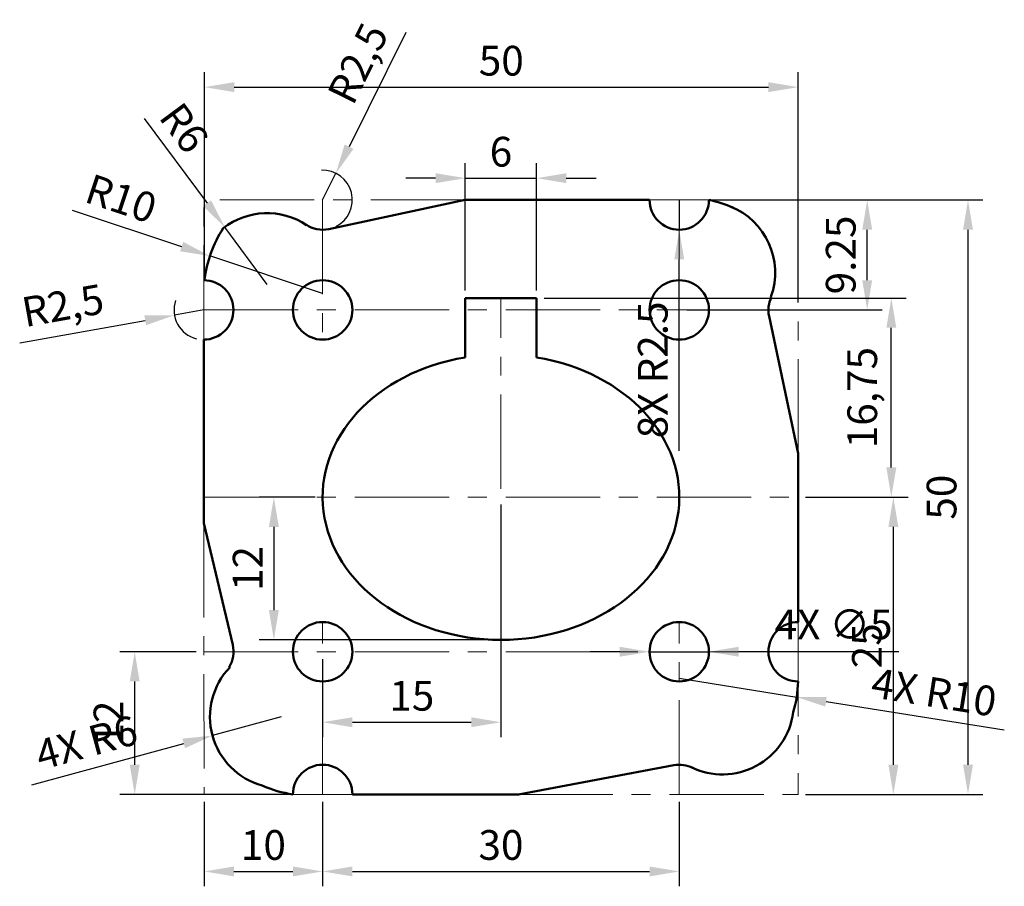
# Model space of a CAD drawing. Units: millimetres. Extents: x 2178 to 2260.8, y 1950.5 to 2023.4.
import ezdxf

# ---------------------------------------------------------------- set-up
doc = ezdxf.new("R2010")
doc.units = ezdxf.units.MM
doc.linetypes.add('CENTER', pattern=[50.8, 31.75, -6.35, 6.35, -6.35])
for name, color, linetype, lineweight in [('M-CNTR', 4, 'CENTER', 18), ('M-CONS', 8, 'CENTER', 13), ('M-DIMS', 2, 'Continuous', 25), ('M-OUTL', 7, 'Continuous', 50)]:
    doc.layers.add(name, color=color, linetype=linetype, lineweight=lineweight)
doc.styles.get("Standard").update_dxf_attribs({"font": 'arial.ttf'})
doc.dimstyles.new('ISO-25', dxfattribs={"dimtxt": 2.5, "dimasz": 2.5, "dimexe": 1.25, "dimexo": 0.625, "dimtad": 1, "dimtxsty": 'Standard', "dimcen": 2.5, "dimadec": 0, "dimazin": 0, "dimtfac": 1, "dimtmove": 0, "dimatfit": 3, "dimfxl": 1, "dimarcsym": 0})

# ---------------------------------------------------------------- blocks, each defined once
blk = doc.blocks.new('*D1')
at = {"layer": 'Defpoints', "color": 0, "transparency": 16777216}
for p in [(2221.441, 2010.03), (2215.441, 1999.949), (2221.441, 1999.949)]:
    blk.add_point(p, dxfattribs=at)
at = {"layer": 'M-DIMS', "color": 0, "lineweight": -2, "transparency": 16777216}
for p, q in [((2215.441, 2000.574), (2215.441, 2011.28)), ((2221.441, 2000.574), (2221.441, 2011.28)), ((2212.941, 2010.03), (2210.441, 2010.03)), ((2215.441, 2010.03), (2221.441, 2010.03)), ((2223.941, 2010.03), (2226.441, 2010.03))]:
    blk.add_line(p, q, dxfattribs=at)
at = {"layer": 'M-DIMS', "color": 0, "transparency": 16777216}
for points in [[(2212.941, 2010.447), (2212.941, 2009.613), (2215.441, 2010.03)], [(2223.941, 2010.447), (2223.941, 2009.613), (2221.441, 2010.03)]]:
    blk.add_solid(points, dxfattribs=at)
at = {"layer": 'M-DIMS', "color": 0, "transparency": 16777216, "insert": (2218.441, 2011.931), "char_height": 2.5, "attachment_point": 5}
blk.add_mtext('6', dxfattribs=at)
blk = doc.blocks.new('*D2')
at = {"layer": 'Defpoints', "color": 0, "transparency": 16777216}
for p in [(2243.441, 2017.687), (2193.504, 2001.448), (2243.441, 1998.949)]:
    blk.add_point(p, dxfattribs=at)
at = {"layer": 'M-DIMS', "color": 0, "lineweight": -2, "transparency": 16777216}
for p, q in [((2193.504, 2002.073), (2193.504, 2018.937)), ((2243.441, 1999.574), (2243.441, 2018.937)), ((2196.004, 2017.687), (2240.941, 2017.687))]:
    blk.add_line(p, q, dxfattribs=at)
at = {"layer": 'M-DIMS', "color": 0, "transparency": 16777216}
for points in [[(2196.004, 2018.104), (2196.004, 2017.27), (2193.504, 2017.687)], [(2240.941, 2018.104), (2240.941, 2017.27), (2243.441, 2017.687)]]:
    blk.add_solid(points, dxfattribs=at)
at = {"layer": 'M-DIMS', "color": 0, "transparency": 16777216, "insert": (2218.472, 2019.588), "char_height": 2.5, "attachment_point": 5}
blk.add_mtext('50', dxfattribs=at)
blk = doc.blocks.new('*D3')
at = {"layer": 'Defpoints', "color": 0, "transparency": 16777216}
for p in [(2203.441, 1983.199), (2199.34, 1971.199), (2218.441, 1971.199)]:
    blk.add_point(p, dxfattribs=at)
at = {"layer": 'M-DIMS', "color": 0, "lineweight": -2, "transparency": 16777216}
for p, q in [((2202.816, 1983.199), (2198.09, 1983.199)), ((2199.34, 1980.699), (2199.34, 1973.699)), ((2217.816, 1971.199), (2198.09, 1971.199))]:
    blk.add_line(p, q, dxfattribs=at)
at = {"layer": 'M-DIMS', "color": 0, "transparency": 16777216}
for points in [[(2198.923, 1980.699), (2199.756, 1980.699), (2199.34, 1983.199)], [(2198.923, 1973.699), (2199.756, 1973.699), (2199.34, 1971.199)]]:
    blk.add_solid(points, dxfattribs=at)
at = {"layer": 'M-DIMS', "color": 0, "transparency": 16777216, "insert": (2197.46, 1977.199), "char_height": 2.5, "attachment_point": 5, "rotation": 90}
blk.add_mtext('12', dxfattribs=at)
blk = doc.blocks.new('*D4')
at = {"layer": 'Defpoints', "color": 0, "transparency": 16777216}
for p in [(2218.441, 1983.199), (2203.441, 1970.199), (2218.441, 1964.27)]:
    blk.add_point(p, dxfattribs=at)
at = {"layer": 'M-DIMS', "color": 0, "lineweight": -2, "transparency": 16777216}
for p, q in [((2218.441, 1982.574), (2218.441, 1963.02)), ((2203.441, 1969.574), (2203.441, 1963.02)), ((2205.941, 1964.27), (2215.941, 1964.27))]:
    blk.add_line(p, q, dxfattribs=at)
at = {"layer": 'M-DIMS', "color": 0, "transparency": 16777216}
for points in [[(2205.941, 1964.687), (2205.941, 1963.853), (2203.441, 1964.27)], [(2215.941, 1964.687), (2215.941, 1963.853), (2218.441, 1964.27)]]:
    blk.add_solid(points, dxfattribs=at)
at = {"layer": 'M-DIMS', "color": 0, "transparency": 16777216, "insert": (2210.941, 1966.171), "char_height": 2.5, "attachment_point": 5}
blk.add_mtext('15', dxfattribs=at)
blk = doc.blocks.new('*D5')
at = {"layer": 'Defpoints', "color": 0, "transparency": 16777216}
for p in [(2193.477, 1958.199), (2203.441, 1958.199), (2203.441, 1951.721)]:
    blk.add_point(p, dxfattribs=at)
at = {"layer": 'M-DIMS', "color": 0, "lineweight": -2, "transparency": 16777216}
for p, q in [((2193.477, 1957.574), (2193.477, 1950.471)), ((2203.441, 1957.574), (2203.441, 1950.471)), ((2195.977, 1951.721), (2200.941, 1951.721))]:
    blk.add_line(p, q, dxfattribs=at)
at = {"layer": 'M-DIMS', "color": 0, "transparency": 16777216}
for points in [[(2195.977, 1952.138), (2195.977, 1951.305), (2193.477, 1951.721)], [(2200.941, 1952.138), (2200.941, 1951.305), (2203.441, 1951.721)]]:
    blk.add_solid(points, dxfattribs=at)
at = {"layer": 'M-DIMS', "color": 0, "transparency": 16777216, "insert": (2198.459, 1953.623), "char_height": 2.5, "attachment_point": 5}
blk.add_mtext('10', dxfattribs=at)
blk = doc.blocks.new('*D6')
at = {"layer": 'Defpoints', "color": 0, "transparency": 16777216}
for p in [(2203.441, 1958.199), (2233.441, 1958.199), (2233.441, 1951.721)]:
    blk.add_point(p, dxfattribs=at)
at = {"layer": 'M-DIMS', "color": 0, "lineweight": -2, "transparency": 16777216}
for p, q in [((2203.441, 1957.574), (2203.441, 1950.471)), ((2233.441, 1957.574), (2233.441, 1950.471)), ((2205.941, 1951.721), (2230.941, 1951.721))]:
    blk.add_line(p, q, dxfattribs=at)
at = {"layer": 'M-DIMS', "color": 0, "transparency": 16777216}
for points in [[(2205.941, 1952.138), (2205.941, 1951.305), (2203.441, 1951.721)], [(2230.941, 1952.138), (2230.941, 1951.305), (2233.441, 1951.721)]]:
    blk.add_solid(points, dxfattribs=at)
at = {"layer": 'M-DIMS', "color": 0, "transparency": 16777216, "insert": (2218.441, 1953.623), "char_height": 2.5, "attachment_point": 5}
blk.add_mtext('30', dxfattribs=at)
blk = doc.blocks.new('*D7')
at = {"layer": 'Defpoints', "color": 0, "transparency": 16777216}
for p in [(2243.441, 1983.199), (2251.45, 1983.199), (2243.441, 1958.199)]:
    blk.add_point(p, dxfattribs=at)
at = {"layer": 'M-DIMS', "color": 0, "lineweight": -2, "transparency": 16777216}
for p, q in [((2244.066, 1983.199), (2252.7, 1983.199)), ((2251.45, 1960.699), (2251.45, 1980.699)), ((2244.066, 1958.199), (2252.7, 1958.199))]:
    blk.add_line(p, q, dxfattribs=at)
at = {"layer": 'M-DIMS', "color": 0, "transparency": 16777216}
for points in [[(2251.033, 1980.699), (2251.867, 1980.699), (2251.45, 1983.199)], [(2251.033, 1960.699), (2251.867, 1960.699), (2251.45, 1958.199)]]:
    blk.add_solid(points, dxfattribs=at)
at = {"layer": 'M-DIMS', "color": 0, "transparency": 16777216, "insert": (2249.549, 1970.699), "char_height": 2.5, "attachment_point": 5, "rotation": 90}
blk.add_mtext('25', dxfattribs=at)
blk = doc.blocks.new('*D8')
at = {"layer": 'Defpoints', "color": 0, "transparency": 16777216}
for p in [(2221.441, 1999.949), (2251.28, 1999.949), (2243.441, 1983.199)]:
    blk.add_point(p, dxfattribs=at)
at = {"layer": 'M-DIMS', "color": 0, "lineweight": -2, "transparency": 16777216}
for p, q in [((2222.066, 1999.949), (2252.53, 1999.949)), ((2251.28, 1985.699), (2251.28, 1997.449)), ((2244.066, 1983.199), (2252.53, 1983.199))]:
    blk.add_line(p, q, dxfattribs=at)
at = {"layer": 'M-DIMS', "color": 0, "transparency": 16777216}
for points in [[(2250.864, 1997.449), (2251.697, 1997.449), (2251.28, 1999.949)], [(2250.864, 1985.699), (2251.697, 1985.699), (2251.28, 1983.199)]]:
    blk.add_solid(points, dxfattribs=at)
at = {"layer": 'M-DIMS', "color": 0, "transparency": 16777216, "insert": (2249.153, 1991.574), "char_height": 2.5, "attachment_point": 5, "rotation": 90}
blk.add_mtext('16,75', dxfattribs=at)
blk = doc.blocks.new('*D9')
at = {"layer": 'Defpoints', "color": 0, "transparency": 16777216}
for p in [(2243.441, 2008.199), (2257.73, 2008.199), (2243.441, 1958.199)]:
    blk.add_point(p, dxfattribs=at)
at = {"layer": 'M-DIMS', "color": 0, "lineweight": -2, "transparency": 16777216}
for p, q in [((2244.066, 2008.199), (2258.98, 2008.199)), ((2257.73, 1960.699), (2257.73, 2005.699)), ((2244.066, 1958.199), (2258.98, 1958.199))]:
    blk.add_line(p, q, dxfattribs=at)
at = {"layer": 'M-DIMS', "color": 0, "transparency": 16777216}
for points in [[(2257.314, 2005.699), (2258.147, 2005.699), (2257.73, 2008.199)], [(2257.314, 1960.699), (2258.147, 1960.699), (2257.73, 1958.199)]]:
    blk.add_solid(points, dxfattribs=at)
at = {"layer": 'M-DIMS', "color": 0, "transparency": 16777216, "insert": (2255.829, 1983.199), "char_height": 2.5, "attachment_point": 5, "rotation": 90}
blk.add_mtext('50', dxfattribs=at)
blk = doc.blocks.new('*D10')
at = {"layer": 'Defpoints', "color": 0, "transparency": 16777216}
for p in [(2193.952, 2003.485), (2203.441, 2000.327)]:
    blk.add_point(p, dxfattribs=at)
at = {"layer": 'M-DIMS', "color": 0, "lineweight": -2, "transparency": 16777216}
for p, q in [((2182.362, 2007.342), (2191.58, 2004.274)), ((2203.441, 2000.327), (2193.952, 2003.485))]:
    blk.add_line(p, q, dxfattribs=at)
at = {"layer": 'M-DIMS', "color": 0, "transparency": 16777216}
blk.add_solid([(2191.712, 2004.67), (2191.449, 2003.879), (2193.952, 2003.485)], dxfattribs=at)
at = {"layer": 'M-DIMS', "color": 0, "transparency": 16777216, "insert": (2186.386, 2008.007), "char_height": 2.5, "attachment_point": 5, "rotation": 341.58983}
blk.add_mtext('R10', dxfattribs=at)
blk = doc.blocks.new('*D11')
at = {"layer": 'Defpoints', "color": 0, "transparency": 16777216}
for p in [(2195.207, 2005.914), (2198.778, 2001.092)]:
    blk.add_point(p, dxfattribs=at)
at = {"layer": 'M-DIMS', "color": 0, "lineweight": -2, "transparency": 16777216}
for p, q in [((2188.433, 2015.06), (2193.719, 2007.923)), ((2198.778, 2001.092), (2195.207, 2005.914))]:
    blk.add_line(p, q, dxfattribs=at)
at = {"layer": 'M-DIMS', "color": 0, "transparency": 16777216}
blk.add_solid([(2194.054, 2008.171), (2193.384, 2007.675), (2195.207, 2005.914)], dxfattribs=at)
at = {"layer": 'M-DIMS', "color": 0, "transparency": 16777216, "insert": (2191.532, 2014.07), "char_height": 2.5, "attachment_point": 5, "rotation": 306.52326}
blk.add_mtext('R6', dxfattribs=at)
blk = doc.blocks.new('*D12')
at = {"layer": 'Defpoints', "color": 0, "transparency": 16777216}
for p in [(2193.441, 1998.949), (2190.979, 1998.51)]:
    blk.add_point(p, dxfattribs=at)
at = {"layer": 'M-DIMS', "color": 0, "lineweight": -2, "transparency": 16777216}
for p, q in [((2193.441, 1998.949), (2190.979, 1998.51)), ((2177.971, 1996.194), (2188.518, 1998.072))]:
    blk.add_line(p, q, dxfattribs=at)
blk.add_arc((2193.441, 1998.949), 2.5, 161.44974, 255.67606, dxfattribs=at)
at = {"layer": 'M-DIMS', "color": 0, "transparency": 16777216}
blk.add_solid([(2188.445, 1998.482), (2188.591, 1997.662), (2190.979, 1998.51)], dxfattribs=at)
at = {"layer": 'M-DIMS', "color": 0, "transparency": 16777216, "insert": (2181.641, 1999.008), "char_height": 2.5, "attachment_point": 5, "rotation": 10.09763}
blk.add_mtext('R2,5', dxfattribs=at)
blk = doc.blocks.new('*D13')
at = {"layer": 'Defpoints', "color": 0, "transparency": 16777216}
for p in [(2204.552, 2010.438), (2203.441, 2008.199)]:
    blk.add_point(p, dxfattribs=at)
at = {"layer": 'M-DIMS', "color": 0, "lineweight": -2, "transparency": 16777216}
for p, q in [((2210.428, 2022.272), (2205.664, 2012.677)), ((2203.441, 2008.199), (2204.552, 2010.438))]:
    blk.add_line(p, q, dxfattribs=at)
blk.add_arc((2203.441, 2008.199), 2.5, 296.34864, 92.24345, dxfattribs=at)
at = {"layer": 'M-DIMS', "color": 0, "transparency": 16777216}
blk.add_solid([(2205.291, 2012.862), (2206.037, 2012.492), (2204.552, 2010.438)], dxfattribs=at)
at = {"layer": 'M-DIMS', "color": 0, "transparency": 16777216, "insert": (2206.697, 2019.54), "char_height": 2.5, "attachment_point": 5, "rotation": 63.59556}
blk.add_mtext('R2,5', dxfattribs=at)
blk = doc.blocks.new('MOUNT-HOLE-D5')
blk.add_circle((2.5, 2.5), 2.5)
blk = doc.blocks.new('*D15')
at = {"layer": 'Defpoints', "color": 0, "transparency": 16777216}
for p in [(2235.941, 2008.199), (2249.251, 2008.199), (2233.441, 1998.949)]:
    blk.add_point(p, dxfattribs=at)
at = {"layer": 'M-DIMS', "color": 0, "lineweight": -2, "transparency": 16777216}
for p, q in [((2236.566, 2008.199), (2250.501, 2008.199)), ((2249.251, 2001.449), (2249.251, 2005.699)), ((2234.066, 1998.949), (2250.501, 1998.949))]:
    blk.add_line(p, q, dxfattribs=at)
at = {"layer": 'M-DIMS', "color": 0, "transparency": 16777216}
for points in [[(2248.834, 2005.699), (2249.667, 2005.699), (2249.251, 2008.199)], [(2248.834, 2001.449), (2249.667, 2001.449), (2249.251, 1998.949)]]:
    blk.add_solid(points, dxfattribs=at)
at = {"layer": 'M-DIMS', "color": 0, "transparency": 16777216, "insert": (2247.349, 2003.574), "char_height": 2.5, "attachment_point": 5, "rotation": 90}
blk.add_mtext('9.25', dxfattribs=at)
blk = doc.blocks.new('*D16')
at = {"layer": 'Defpoints', "color": 0, "transparency": 16777216}
for p in [(2187.631, 1970.199), (2193.441, 1970.199), (2200.941, 1958.199)]:
    blk.add_point(p, dxfattribs=at)
at = {"layer": 'M-DIMS', "color": 0, "lineweight": -2, "transparency": 16777216}
for p, q in [((2192.816, 1970.199), (2186.381, 1970.199)), ((2187.631, 1960.699), (2187.631, 1967.699)), ((2200.316, 1958.199), (2186.381, 1958.199))]:
    blk.add_line(p, q, dxfattribs=at)
at = {"layer": 'M-DIMS', "color": 0, "transparency": 16777216}
for points in [[(2187.214, 1967.699), (2188.047, 1967.699), (2187.631, 1970.199)], [(2187.214, 1960.699), (2188.047, 1960.699), (2187.631, 1958.199)]]:
    blk.add_solid(points, dxfattribs=at)
at = {"layer": 'M-DIMS', "color": 0, "transparency": 16777216, "insert": (2185.75, 1964.199), "char_height": 2.5, "attachment_point": 5, "rotation": 90}
blk.add_mtext('12', dxfattribs=at)
blk = doc.blocks.new('*D17')
at = {"layer": 'Defpoints', "color": 0, "transparency": 16777216}
for p in [(2233.444, 1967.971), (2243.319, 1966.391)]:
    blk.add_point(p, dxfattribs=at)
at = {"layer": 'M-DIMS', "color": 0, "lineweight": -2, "transparency": 16777216}
for p, q in [((2233.444, 1967.971), (2243.319, 1966.391)), ((2260.784, 1963.596), (2245.787, 1965.996))]:
    blk.add_line(p, q, dxfattribs=at)
at = {"layer": 'M-DIMS', "color": 0, "transparency": 16777216}
blk.add_solid([(2245.853, 1966.407), (2245.721, 1965.585), (2243.319, 1966.391)], dxfattribs=at)
at = {"layer": 'M-DIMS', "color": 0, "transparency": 16777216, "insert": (2254.82, 1966.476), "char_height": 2.5, "attachment_point": 5, "rotation": 350.90899}
blk.add_mtext('4X R10', dxfattribs=at)
blk = doc.blocks.new('*D18')
at = {"layer": 'Defpoints', "color": 0, "transparency": 16777216}
for p in [(2199.959, 1964.726), (2194.17, 1963.149)]:
    blk.add_point(p, dxfattribs=at)
at = {"layer": 'M-DIMS', "color": 0, "lineweight": -2, "transparency": 16777216}
for p, q in [((2199.959, 1964.726), (2194.17, 1963.149)), ((2178.972, 1959.009), (2191.758, 1962.492))]:
    blk.add_line(p, q, dxfattribs=at)
at = {"layer": 'M-DIMS', "color": 0, "transparency": 16777216}
blk.add_solid([(2191.648, 1962.894), (2191.867, 1962.09), (2194.17, 1963.149)], dxfattribs=at)
at = {"layer": 'M-DIMS', "color": 0, "transparency": 16777216, "insert": (2183.659, 1962.257), "char_height": 2.5, "attachment_point": 5, "rotation": 15.23757}
blk.add_mtext('4X R6', dxfattribs=at)
blk = doc.blocks.new('*D19')
at = {"layer": 'Defpoints', "color": 0, "transparency": 16777216}
for p in [(2233.441, 2008.199), (2233.44, 2005.699)]:
    blk.add_point(p, dxfattribs=at)
at = {"layer": 'M-DIMS', "color": 0, "lineweight": -2, "transparency": 16777216}
for p, q in [((2233.441, 2008.199), (2233.44, 2005.699)), ((2233.436, 1987.111), (2233.439, 2003.199))]:
    blk.add_line(p, q, dxfattribs=at)
at = {"layer": 'M-DIMS', "color": 0, "transparency": 16777216}
blk.add_solid([(2233.023, 2003.199), (2233.856, 2003.199), (2233.44, 2005.699)], dxfattribs=at)
at = {"layer": 'M-DIMS', "color": 0, "transparency": 16777216, "insert": (2231.536, 1993.905), "char_height": 2.5, "attachment_point": 5, "rotation": 89.98728}
blk.add_mtext('8X R2.5', dxfattribs=at)
blk = doc.blocks.new('*D20')
at = {"layer": 'Defpoints', "color": 0, "transparency": 16777216}
for p in [(2230.941, 1970.198), (2235.941, 1970.199)]:
    blk.add_point(p, dxfattribs=at)
at = {"layer": 'M-DIMS', "color": 0, "lineweight": -2, "transparency": 16777216}
for p, q in [((2228.441, 1970.198), (2225.941, 1970.198)), ((2230.941, 1970.198), (2235.941, 1970.199)), ((2251.907, 1970.201), (2238.441, 1970.199))]:
    blk.add_line(p, q, dxfattribs=at)
at = {"layer": 'M-DIMS', "color": 0, "transparency": 16777216}
for points in [[(2228.44, 1970.615), (2228.441, 1969.781), (2230.941, 1970.198)], [(2238.44, 1970.616), (2238.441, 1969.783), (2235.941, 1970.199)]]:
    blk.add_solid(points, dxfattribs=at)
at = {"layer": 'M-DIMS', "color": 0, "transparency": 16777216, "insert": (2246.424, 1972.172), "char_height": 2.5, "attachment_point": 5, "rotation": 0.00846}
blk.add_mtext('4X ∅5', dxfattribs=at)

msp = doc.modelspace()

# ---------------------------------------------------------------- linework, layer by layer
at = {"layer": 'M-CNTR', "ltscale": 0.25, "transparency": 33554534}
for p, q in [((2203.441, 2008.199), (2203.441, 1996.449)), ((2233.441, 2008.199), (2233.441, 1996.449)), ((2218.441, 1971.199), (2218.441, 1999.949)), ((2193.441, 1998.949), (2243.441, 1998.949)), ((2193.441, 1983.199), (2243.441, 1983.199)), ((2203.441, 1958.199), (2203.441, 1972.699)), ((2233.441, 1958.199), (2233.441, 1972.699)), ((2193.441, 1970.199), (2243.441, 1970.199))]:
    msp.add_line(p, q, dxfattribs=at)
at = {"layer": 'M-CONS', "ltscale": 0.25, "transparency": 33554534}
for p, q in [((2215.441, 2008.199), (2193.441, 2008.199)), ((2193.441, 1996.449), (2193.441, 2008.199)), ((2230.941, 2008.199), (2243.441, 2008.199)), ((2243.441, 1986.865), (2243.441, 2008.199)), ((2193.441, 1981.023), (2193.477, 1958.199)), ((2243.441, 1972.699), (2243.441, 1958.199)), ((2205.941, 1958.199), (2193.477, 1958.199)), ((2219.91, 1958.199), (2243.441, 1958.199))]:
    msp.add_line(p, q, dxfattribs=at)
at = {"layer": 'M-CONS'}
msp.add_line((2203.441, 1972.699), (2203.441, 1972.699), dxfattribs=at)
at = {"layer": 'M-OUTL'}
for p, q in [((2215.441, 2008.199), (2203.961, 2005.753)), ((2215.441, 2008.199), (2230.941, 2008.199)), ((2218.441, 1999.949), (2215.441, 1999.949)), ((2215.441, 1994.956), (2215.441, 1999.949)), ((2218.441, 1999.949), (2221.441, 1999.949)), ((2221.441, 1994.956), (2221.441, 1999.949)), ((2241.185, 2000.026), (2241.153, 2000.057)), ((2243.441, 1986.865), (2240.995, 1998.431)), ((2193.441, 1981.023), (2193.441, 1996.449)), ((2243.441, 1986.865), (2243.441, 1972.699)), ((2193.441, 1981.023), (2195.873, 1970.776)), ((2195.649, 1968.9), (2195.577, 1968.9)), ((2219.91, 1958.199), (2232.979, 1960.656)), ((2219.91, 1958.199), (2205.941, 1958.199))]:
    msp.add_line(p, q, dxfattribs=at)
for centre, radius, start, end in [((2233.441, 2008.199), 2.5, 180, 0), ((2233.944, 1998.4), 10, 66.30105, 78.48355), ((2198.778, 2001.092), 6, 56.43501, 127.97367), ((2235.506, 2002.083), 6, 340.26737, 68.22658), ((2203.441, 2008.199), 2.5, 236.02305, 282.0247), ((2203.441, 2000.327), 10, 146.66495, 173.56187), ((2193.441, 1998.949), 2.5, 270, 90), ((2243.441, 1998.949), 2.5, 154.47105, 191.94004), ((2243.441, 1970.199), 2.5, 90, 270), ((2193.441, 1970.199), 2.5, 328.71421, 13.35305), ((2199.959, 1964.726), 6, 135.91386, 254.57022), ((2233.444, 1967.971), 10, 343.37782, 358.43874), ((2237.076, 1965.88), 6, 243.88082, 352.63297), ((2203.441, 1958.199), 2.5, 0, 180), ((2233.441, 1958.199), 2.5, 62.77181, 100.6478), ((2202.398, 1968.092), 10, 246.20101, 261.61958)]:
    msp.add_arc(centre, radius, start, end, dxfattribs=at)
msp.add_ellipse((2218.441, 1983.199), major_axis=(15, 0), ratio=0.8, start_param=1.772154, end_param=7.652624, dxfattribs=at)

# ---------------------------------------------------------------- block references
for p in [(2200.941, 1996.449), (2230.941, 1996.449), (2200.941, 1967.699), (2230.941, 1967.699)]:
    msp.add_blockref('MOUNT-HOLE-D5', p, dxfattribs=at)

# ---------------------------------------------------------------- dimensions: what is measured, and where the dimension line sits
at = {"layer": 'M-DIMS'}
for center, mpoint, picture, middle in [((2203.441, 2008.199), (2204.552, 2010.438), '*D13', (2206.697, 2019.54)), ((2203.441, 2000.327), (2193.952, 2003.485), '*D10', (2186.386, 2008.007)), ((2193.441, 1998.949), (2190.979, 1998.51), '*D12', (2181.641, 1999.008))]:
    dim = msp.add_radius_dim(center=center, mpoint=mpoint, dimstyle='ISO-25', override={"dimclrd": 0, "dimclre": 0, "dimclrt": 0}, dxfattribs=at)
    dim.commit()
    dim.dimension.update_dxf_attribs({"geometry": picture, "text_midpoint": middle})
for base, p1, p2, override, picture, middle in [((2243.441, 2017.687), (2193.504, 2001.448), (2243.441, 1998.949), {"dimdec": 0, "dimclrd": 0, "dimclre": 0, "dimclrt": 0}, '*D2', (2218.472, 2019.588)), ((2221.441, 2010.03), (2215.441, 1999.949), (2221.441, 1999.949), {"dimclrd": 0, "dimclre": 0, "dimclrt": 0}, '*D1', (2218.441, 2011.931)), ((2218.441, 1964.27), (2203.441, 1970.199), (2218.441, 1983.199), {"dimclrd": 0, "dimclre": 0, "dimclrt": 0}, '*D4', (2210.941, 1966.171)), ((2203.441, 1951.721), (2193.477, 1958.199), (2203.441, 1958.199), {"dimdec": 0, "dimclrd": 0, "dimclre": 0, "dimclrt": 0}, '*D5', (2198.459, 1953.623)), ((2233.441, 1951.721), (2203.441, 1958.199), (2233.441, 1958.199), {"dimclrd": 0, "dimclre": 0, "dimclrt": 0}, '*D6', (2218.441, 1953.623))]:
    dim = msp.add_linear_dim(base=base, p1=p1, p2=p2, dimstyle='ISO-25', override=override, dxfattribs=at)
    dim.commit()
    dim.dimension.update_dxf_attribs({"geometry": picture, "text_midpoint": middle})
dim = msp.add_radius_dim(center=(2198.778, 2001.092), mpoint=(2195.207, 2005.914), dimstyle='ISO-25', override={"dimclrd": 0, "dimclre": 0, "dimclrt": 0}, dxfattribs=at)
dim.commit()
dim.dimension.update_dxf_attribs({"geometry": '*D11', "text_midpoint": (2190.004, 2012.939), "dimtype": 164})
for center, mpoint, text, override, picture, middle in [((2233.441, 2008.199), (2233.44, 2005.699), '8X <>', {"dimdec": 1, "dimlfac": 1, "dimrnd": 0, "dimzin": 0, "dimdsep": 46, "dimlunit": 2}, '*D19', (2231.536, 1993.905)), ((2233.444, 1967.971), (2243.319, 1966.391), '4X <>', {"dimdec": 0, "dimlfac": 1, "dimrnd": 0, "dimzin": 0, "dimdsep": 46, "dimlunit": 2}, '*D17', (2254.82, 1966.476)), ((2199.959, 1964.726), (2194.17, 1963.149), '4X <>', {"dimdec": 0, "dimlfac": 1, "dimrnd": 0, "dimzin": 0, "dimdsep": 46, "dimlunit": 2}, '*D18', (2183.659, 1962.257))]:
    dim = msp.add_radius_dim(center=center, mpoint=mpoint, text=text, dimstyle='ISO-25', override=override, dxfattribs=at)
    dim.commit()
    dim.dimension.update_dxf_attribs({"geometry": picture, "text_midpoint": middle})
for base, p1, p2, override, picture, middle in [((2249.251, 2008.199), (2233.441, 1998.949), (2235.941, 2008.199), {"dimdec": 2, "dimlfac": 1, "dimrnd": 0, "dimzin": 0, "dimdsep": 46, "dimlunit": 2}, '*D15', (2247.349, 2003.574)), ((2257.73, 2008.199), (2243.441, 1958.199), (2243.441, 2008.199), {"dimclrd": 0, "dimclre": 0, "dimclrt": 0}, '*D9', (2255.829, 1983.199)), ((2251.28, 1999.949), (2243.441, 1983.199), (2221.441, 1999.949), {"dimclrd": 0, "dimclre": 0, "dimclrt": 0}, '*D8', (2249.153, 1991.574)), ((2199.34, 1971.199), (2203.441, 1983.199), (2218.441, 1971.199), {"dimclrd": 0, "dimclre": 0, "dimclrt": 0}, '*D3', (2197.46, 1977.199)), ((2251.45, 1983.199), (2243.441, 1958.199), (2243.441, 1983.199), {"dimclrd": 0, "dimclre": 0, "dimclrt": 0}, '*D7', (2249.549, 1970.699)), ((2187.631, 1970.199), (2200.941, 1958.199), (2193.441, 1970.199), {"dimdec": 0, "dimlfac": 1, "dimrnd": 0, "dimzin": 0, "dimdsep": 46, "dimlunit": 2}, '*D16', (2185.75, 1964.199))]:
    dim = msp.add_linear_dim(base=base, p1=p1, p2=p2, angle=90, dimstyle='ISO-25', override=override, dxfattribs=at)
    dim.commit()
    dim.dimension.update_dxf_attribs({"geometry": picture, "text_midpoint": middle})
dim = msp.add_diameter_dim_2p(p1=(2230.941, 1970.198), p2=(2235.941, 1970.199), text='4X <>', dimstyle='ISO-25', override={"dimdec": 0, "dimlfac": 1, "dimrnd": 0, "dimzin": 0, "dimdsep": 46, "dimlunit": 2}, dxfattribs=at)
dim.commit()
dim.dimension.update_dxf_attribs({"geometry": '*D20', "text_midpoint": (2246.424, 1970.201), "dimtype": 163})

doc.saveas('drawing.dxf')
